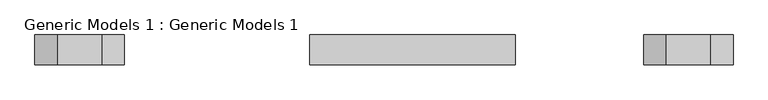
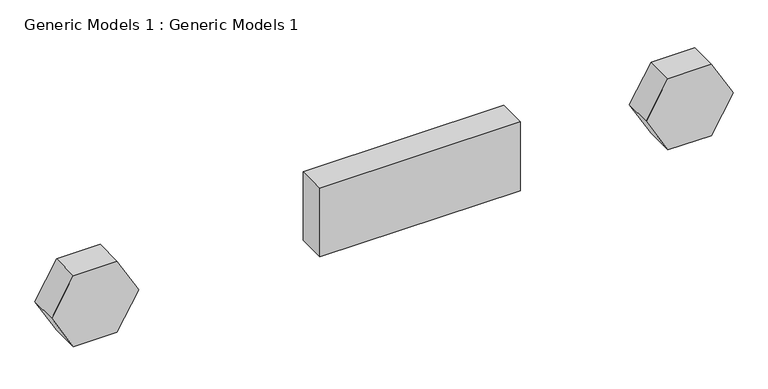
"""IFC4 building model written with IfcOpenShell, lengths in millimetres: proxy geometry, Generic Models 1 : Generic Models 1."""

from ifc_helpers import new_model, si_unit, frame, origin, place, context, project, spatial, polyline, outline, extrude, source, transform, mapped, element, save


def generic_models_1_generic_models_1_074ece3c(model_context):
    return source(origin(), model_context, "Body", "SweptSolid", [
        extrude(outline(polyline([(-136.1449167, -5927.3570853), (-2244.3449167, -5927.3570853), (-2244.3449167, -5622.5570853), (-136.1449167, -5622.5570853), (-136.1449167, -5927.3570853)])), frame((0.0, 0.0, 9884.3380145), z_axis=(0.0, 0.0, 1.0), x_axis=(1.0, 0.0, 0.0)), (0.0, 0.0, 1.0), 762.0),
        extrude(outline(polyline([(10585.0848291, -4377.9449167), (10585.0848291, -4835.1449167), (10189.1380145, -5063.7449167), (9793.1911999, -4835.1449167), (9793.1911999, -4377.9449167), (10189.1380145, -4149.3449167), (10585.0848291, -4377.9449167)])), frame((0.0, -5927.3570853, 0.0), z_axis=(0.0, 1.0, 0.0), x_axis=(0.0, 0.0, 1.0)), (0.0, 0.0, 1.0), 304.8),
        extrude(outline(polyline([(10585.0848291, 1870.4550833), (10585.0848291, 1413.2550833), (10189.1380145, 1184.6550833), (9793.1911999, 1413.2550833), (9793.1911999, 1870.4550833), (10189.1380145, 2099.0550833), (10585.0848291, 1870.4550833)])), frame((0.0, -5927.3570853, 0.0), z_axis=(0.0, 1.0, 0.0), x_axis=(0.0, 0.0, 1.0)), (0.0, 0.0, 1.0), 304.8),
    ])


if __name__ == "__main__":
    model = new_model("IFC4")
    model_context = context("Model", 3, world=origin())
    ifc_project = project(units=[si_unit("LENGTHUNIT", "METRE", prefix="MILLI")], contexts=[model_context])
    site = spatial("IfcSite", under=ifc_project)
    building = spatial("IfcBuilding", under=site)
    placement = place(None, origin())
    generic_models_1_generic_models_1_shape = generic_models_1_generic_models_1_074ece3c(model_context)
    element("IfcBuildingElementProxy", 1, Name="Generic Models 1 : Generic Models 1", ObjectType="Generic Models 1 : Generic Models 1", at=placement, inside=building, context=model_context, shape_type="MappedRepresentation", body=[
        mapped(generic_models_1_generic_models_1_shape, transform((0.0, 0.0, 0.0), x_axis=(1.0, 0.0, 0.0), y_axis=(0.0, 1.0, 0.0), z_axis=(0.0, 0.0, 1.0))),
    ])
    save(model, "model.ifc")

# Revit data of these elements
# Element 1 (IfcBuildingElementProxy, "Generic Models 1 : Generic Models 1")
#   Materials on its faces: "Parking Stripe"
# Materials
#   "Parking Stripe": class "Paint", colour RGB 250 250 91, transparency 0, Cost = 0
